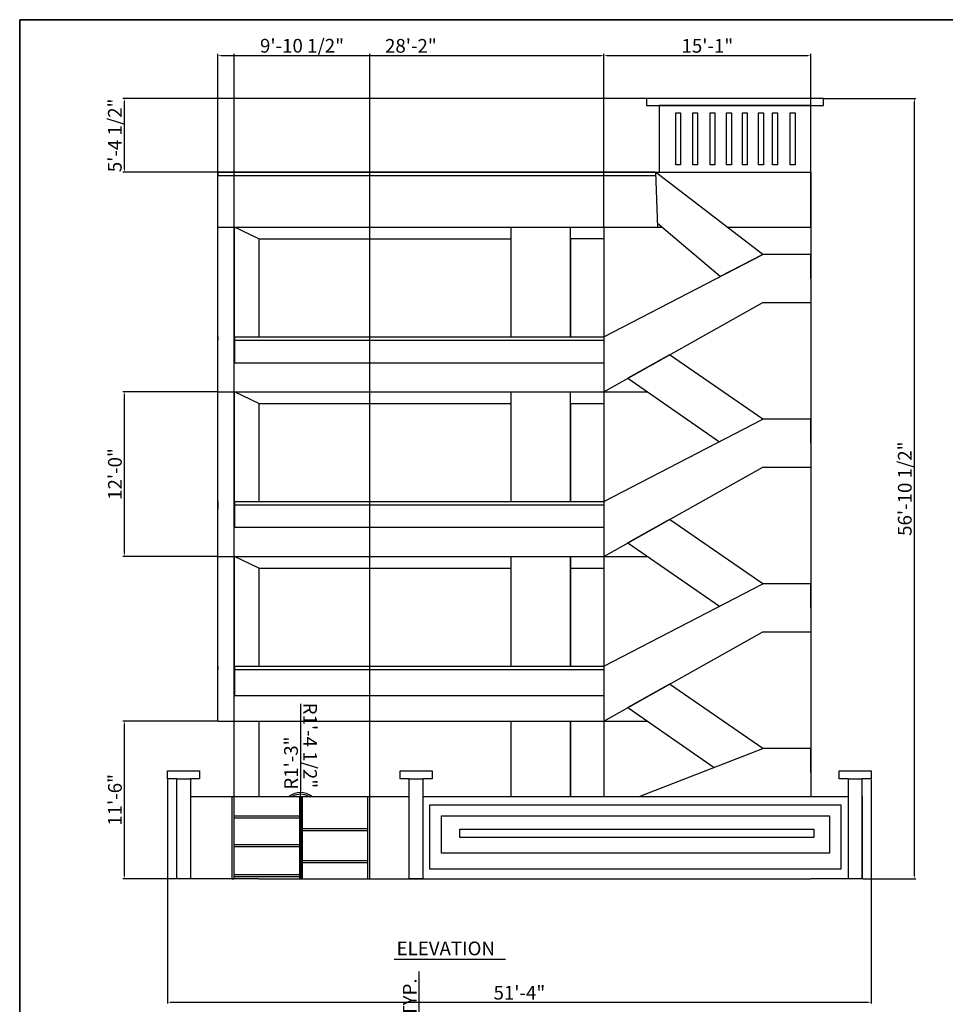
# Model space of a CAD drawing. Units: inches. Extents: x 1266 to 2869, y -408 to 3241.
# Tile 10 of 11: x 1266 to 2076, y 2380 to 3241. Entities that reach past the tile are written whole.
import ezdxf

# ---------------------------------------------------------------- set-up
doc = ezdxf.new("R2010")
doc.units = ezdxf.units.IN
for name, color, linetype, lineweight in [('A-ANNO-DIMS', 2, 'Continuous', 18), ('A-ANNO-TITL', 7, 'Continuous', 25), ('A-ANNO-TTLB', 7, 'Continuous', 35), ('A-ELEV', 7, 'Continuous', 25), ('A-ELEV-GATE', 7, 'Continuous', 25)]:
    doc.layers.add(name, color=color, linetype=linetype, lineweight=lineweight)
doc.styles.get("Standard").update_dxf_attribs({"font": 'arial.ttf'})
doc.dimstyles.new('ISO-25', dxfattribs={"dimtxt": 12, "dimasz": 2.5, "dimexe": 1.25, "dimexo": 0.625, "dimtad": 1, "dimdec": 0, "dimlunit": 3, "dimtxsty": 'Standard', "dimcen": 2.5, "dimadec": 0, "dimazin": 0, "dimtfac": 1, "dimtdec": 0, "dimtmove": 0, "dimatfit": 3, "dimfxl": 1, "dimarcsym": 0})

# ---------------------------------------------------------------- blocks, each defined once
blk = doc.blocks.new('*D53')
at = {"layer": 'A-ANNO-DIMS', "color": 0, "lineweight": -2, "transparency": 16777216}
for p, q in [((1616.02, 2184.29), (1616.02, 2408.76)), ((1611.05, 2184.29), (1617.27, 2184.29)), ((1616.02, 2149.49), (1616.02, 2181.79)), ((1611.05, 2146.99), (1617.27, 2146.99))]:
    blk.add_line(p, q, dxfattribs=at)
at = {"layer": 'A-ANNO-DIMS', "color": 0, "transparency": 16777216}
for points in [[(1615.6, 2181.79), (1616.43, 2181.79), (1616.02, 2184.29)], [(1615.6, 2149.49), (1616.43, 2149.49), (1616.02, 2146.99)]]:
    blk.add_solid(points, dxfattribs=at)
at = {"layer": 'Defpoints', "color": 0, "transparency": 16777216}
for p in [(1610.42, 2184.29), (1616.02, 2184.29), (1610.42, 2146.99)]:
    blk.add_point(p, dxfattribs=at)
at = {"layer": 'A-ANNO-DIMS', "color": 0, "transparency": 16777216, "insert": (1609.18, 2297.78), "char_height": 12, "attachment_point": 5, "rotation": 90}
blk.add_mtext('BEDROOM DR 3\'-1 1/2" TYP.', dxfattribs=at)
blk = doc.blocks.new('*D88')
at = {"layer": 'A-ANNO-DIMS', "color": 0, "lineweight": -2, "transparency": 16777216}
for p, q in [((1395.69, 2576.89), (1395.69, 2380.74)), ((2011.5, 2576.89), (2011.5, 2380.74)), ((1398.19, 2381.99), (2009, 2381.99))]:
    blk.add_line(p, q, dxfattribs=at)
at = {"layer": 'A-ANNO-DIMS', "color": 0, "transparency": 16777216}
for points in [[(1398.19, 2382.41), (1398.19, 2381.57), (1395.69, 2381.99)], [(2009, 2382.41), (2009, 2381.57), (2011.5, 2381.99)]]:
    blk.add_solid(points, dxfattribs=at)
at = {"layer": 'Defpoints', "color": 0, "transparency": 16777216}
for p in [(1395.69, 2577.52), (2011.5, 2577.52), (2011.5, 2381.99)]:
    blk.add_point(p, dxfattribs=at)
at = {"layer": 'A-ANNO-DIMS', "color": 0, "transparency": 16777216, "insert": (1703.6, 2388.74), "char_height": 12, "attachment_point": 5}
blk.add_mtext('51\'-4"', dxfattribs=at)
blk = doc.blocks.new('*D89')
at = {"layer": 'A-ANNO-DIMS', "color": 0, "lineweight": -2, "transparency": 16777216}
for p, q in [((1970.49, 3172.35), (2050.55, 3172.35)), ((2049.3, 2492.46), (2049.3, 3169.85)), ((2004.13, 2489.96), (2050.55, 2489.96))]:
    blk.add_line(p, q, dxfattribs=at)
at = {"layer": 'A-ANNO-DIMS', "color": 0, "transparency": 16777216}
for points in [[(2048.89, 3169.85), (2049.72, 3169.85), (2049.3, 3172.35)], [(2048.89, 2492.46), (2049.72, 2492.46), (2049.3, 2489.96)]]:
    blk.add_solid(points, dxfattribs=at)
at = {"layer": 'Defpoints', "color": 0, "transparency": 16777216}
for p in [(1969.86, 3172.35), (2049.3, 3172.35), (2003.5, 2489.96)]:
    blk.add_point(p, dxfattribs=at)
at = {"layer": 'A-ANNO-DIMS', "color": 0, "transparency": 16777216, "insert": (2042.47, 2831.15), "char_height": 12, "attachment_point": 5, "rotation": 90}
blk.add_mtext('56\'-10 1/2"', dxfattribs=at)
blk = doc.blocks.new('*D90')
at = {"layer": 'A-ANNO-DIMS', "color": 0, "lineweight": -2, "transparency": 16777216}
for p, q in [((1439.69, 3108.58), (1439.69, 3211.4)), ((1442.19, 3210.15), (1775.05, 3210.15)), ((1777.55, 3060.58), (1777.55, 3211.4))]:
    blk.add_line(p, q, dxfattribs=at)
at = {"layer": 'A-ANNO-DIMS', "color": 0, "transparency": 16777216}
for points in [[(1442.19, 3210.57), (1442.19, 3209.73), (1439.69, 3210.15)], [(1775.05, 3210.57), (1775.05, 3209.73), (1777.55, 3210.15)]]:
    blk.add_solid(points, dxfattribs=at)
at = {"layer": 'Defpoints', "color": 0, "transparency": 16777216}
for p in [(1777.55, 3210.15), (1439.69, 3107.96), (1777.55, 3059.96)]:
    blk.add_point(p, dxfattribs=at)
at = {"layer": 'A-ANNO-DIMS', "color": 0, "transparency": 16777216, "insert": (1608.62, 3216.9), "char_height": 12, "attachment_point": 5}
blk.add_mtext('28\'-2"', dxfattribs=at)
blk = doc.blocks.new('*D91')
at = {"layer": 'A-ANNO-DIMS', "color": 0, "lineweight": -2, "transparency": 16777216}
for p, q in [((1777.55, 3060.58), (1777.55, 3211.4)), ((1780.05, 3210.15), (1956.19, 3210.15)), ((1958.69, 3060.58), (1958.69, 3211.4))]:
    blk.add_line(p, q, dxfattribs=at)
at = {"layer": 'A-ANNO-DIMS', "color": 0, "transparency": 16777216}
for points in [[(1780.05, 3210.57), (1780.05, 3209.73), (1777.55, 3210.15)], [(1956.19, 3210.57), (1956.19, 3209.73), (1958.69, 3210.15)]]:
    blk.add_solid(points, dxfattribs=at)
at = {"layer": 'Defpoints', "color": 0, "transparency": 16777216}
for p in [(1958.69, 3210.15), (1777.55, 3059.96), (1958.69, 3059.96)]:
    blk.add_point(p, dxfattribs=at)
at = {"layer": 'A-ANNO-DIMS', "color": 0, "transparency": 16777216, "insert": (1868.12, 3216.9), "char_height": 12, "attachment_point": 5}
blk.add_mtext('15\'-1"', dxfattribs=at)
blk = doc.blocks.new('*D92')
at = {"layer": 'A-ANNO-DIMS', "color": 0, "lineweight": -2, "transparency": 16777216}
for p, q in [((1439.07, 2915.96), (1356.64, 2915.96)), ((1357.89, 2774.46), (1357.89, 2913.46)), ((1439.07, 2771.96), (1356.64, 2771.96))]:
    blk.add_line(p, q, dxfattribs=at)
at = {"layer": 'A-ANNO-DIMS', "color": 0, "transparency": 16777216}
for points in [[(1357.48, 2913.46), (1358.31, 2913.46), (1357.89, 2915.96)], [(1357.48, 2774.46), (1358.31, 2774.46), (1357.89, 2771.96)]]:
    blk.add_solid(points, dxfattribs=at)
at = {"layer": 'Defpoints', "color": 0, "transparency": 16777216}
for p in [(1357.89, 2915.96), (1439.69, 2915.96), (1439.69, 2771.96)]:
    blk.add_point(p, dxfattribs=at)
at = {"layer": 'A-ANNO-DIMS', "color": 0, "transparency": 16777216, "insert": (1351.14, 2843.96), "char_height": 12, "attachment_point": 5, "rotation": 90}
blk.add_mtext('12\'-0"', dxfattribs=at)
blk = doc.blocks.new('*D93')
at = {"layer": 'A-ANNO-DIMS', "color": 0, "lineweight": -2, "transparency": 16777216}
for p, q in [((1969.24, 3172.35), (1356.64, 3172.35)), ((1357.89, 3110.46), (1357.89, 3169.85)), ((1822.02, 3107.96), (1356.64, 3107.96))]:
    blk.add_line(p, q, dxfattribs=at)
at = {"layer": 'A-ANNO-DIMS', "color": 0, "transparency": 16777216}
for points in [[(1357.48, 3169.85), (1358.31, 3169.85), (1357.89, 3172.35)], [(1357.48, 3110.46), (1358.31, 3110.46), (1357.89, 3107.96)]]:
    blk.add_solid(points, dxfattribs=at)
at = {"layer": 'Defpoints', "color": 0, "transparency": 16777216}
for p in [(1357.89, 3172.35), (1969.86, 3172.35), (1822.65, 3107.96)]:
    blk.add_point(p, dxfattribs=at)
at = {"layer": 'A-ANNO-DIMS', "color": 0, "transparency": 16777216, "insert": (1351.06, 3140.15), "char_height": 12, "attachment_point": 5, "rotation": 90}
blk.add_mtext('5\'-4 1/2"', dxfattribs=at)
blk = doc.blocks.new('*D94')
at = {"layer": 'A-ANNO-DIMS', "color": 0, "lineweight": -2, "transparency": 16777216}
for p, q in [((1439.07, 2627.96), (1356.64, 2627.96)), ((1357.89, 2492.46), (1357.89, 2625.46)), ((1403.07, 2489.96), (1356.64, 2489.96))]:
    blk.add_line(p, q, dxfattribs=at)
at = {"layer": 'A-ANNO-DIMS', "color": 0, "transparency": 16777216}
for points in [[(1357.48, 2625.46), (1358.31, 2625.46), (1357.89, 2627.96)], [(1357.48, 2492.46), (1358.31, 2492.46), (1357.89, 2489.96)]]:
    blk.add_solid(points, dxfattribs=at)
at = {"layer": 'Defpoints', "color": 0, "transparency": 16777216}
for p in [(1357.89, 2627.96), (1439.69, 2627.96), (1403.69, 2489.96)]:
    blk.add_point(p, dxfattribs=at)
at = {"layer": 'A-ANNO-DIMS', "color": 0, "transparency": 16777216, "insert": (1351.14, 2558.96), "char_height": 12, "attachment_point": 5, "rotation": 90}
blk.add_mtext('11\'-6"', dxfattribs=at)
blk = doc.blocks.new('*D95')
at = {"layer": 'A-ANNO-DIMS', "color": 0, "lineweight": -2, "transparency": 16777216}
for p, q in [((1454.05, 2562.58), (1454.05, 3211.4)), ((1456.55, 3210.15), (1570.14, 3210.15)), ((1572.64, 2562.58), (1572.64, 3211.4))]:
    blk.add_line(p, q, dxfattribs=at)
at = {"layer": 'A-ANNO-DIMS', "color": 0, "transparency": 16777216}
for points in [[(1456.55, 3210.57), (1456.55, 3209.73), (1454.05, 3210.15)], [(1570.14, 3210.57), (1570.14, 3209.73), (1572.64, 3210.15)]]:
    blk.add_solid(points, dxfattribs=at)
at = {"layer": 'Defpoints', "color": 0, "transparency": 16777216}
for p in [(1572.64, 3210.15), (1454.05, 2561.96), (1572.64, 2561.96)]:
    blk.add_point(p, dxfattribs=at)
at = {"layer": 'A-ANNO-DIMS', "color": 0, "transparency": 16777216, "insert": (1513.34, 3216.98), "char_height": 12, "attachment_point": 5}
blk.add_mtext('9\'-10 1/2"', dxfattribs=at)
blk = doc.blocks.new('*D102')
at = {"layer": 'A-ANNO-DIMS', "color": 0, "lineweight": -2, "transparency": 16777216}
for p, q in [((1512.02, 2642.88), (1512.02, 2567.79)), ((1512.02, 2548.71), (1512.02, 2565.29))]:
    blk.add_line(p, q, dxfattribs=at)
at = {"layer": 'A-ANNO-DIMS', "color": 0, "transparency": 16777216}
blk.add_solid([(1512.44, 2567.79), (1511.61, 2567.79), (1512.02, 2565.29)], dxfattribs=at)
at = {"layer": 'Defpoints', "color": 0, "transparency": 16777216}
for p in [(1512.02, 2565.29), (1512.02, 2548.71)]:
    blk.add_point(p, dxfattribs=at)
at = {"layer": 'A-ANNO-DIMS', "color": 0, "transparency": 16777216, "insert": (1518.85, 2606.59), "char_height": 12, "attachment_point": 5, "rotation": 270.00131}
blk.add_mtext('R1\'-4 1/2"', dxfattribs=at)
blk = doc.blocks.new('*D103')
at = {"layer": 'A-ANNO-DIMS', "color": 0, "lineweight": -2, "transparency": 16777216}
for p, q in [((1512.08, 2613.48), (1512.08, 2566.34)), ((1512.08, 2548.82), (1512.08, 2563.84))]:
    blk.add_line(p, q, dxfattribs=at)
at = {"layer": 'A-ANNO-DIMS', "color": 0, "transparency": 16777216}
blk.add_solid([(1511.66, 2566.34), (1512.49, 2566.34), (1512.08, 2563.84)], dxfattribs=at)
at = {"layer": 'Defpoints', "color": 0, "transparency": 16777216}
for p in [(1512.08, 2563.84), (1512.08, 2548.82)]:
    blk.add_point(p, dxfattribs=at)
at = {"layer": 'A-ANNO-DIMS', "color": 0, "transparency": 16777216, "insert": (1505.32, 2591.16), "char_height": 12, "attachment_point": 5, "rotation": 89.99844}
blk.add_mtext('R1\'-3"', dxfattribs=at)

msp = doc.modelspace()

# ---------------------------------------------------------------- linework, layer by layer
at = {"layer": 'A-ANNO-TITL'}
msp.add_line((1594.11, 2419.79), (1691.47, 2419.79), dxfattribs=at)
at = {"layer": 'A-ANNO-TTLB'}
msp.add_lwpolyline([(1266.23, 3241.34), (2868.62, 3241.34), (2868.62, 986.84), (1266.23, 986.84)], close=True, dxfattribs=at)
at = {"layer": 'A-ELEV'}
for p, q in [((1969.86, 3172.35), (1814.99, 3172.35)), ((1814.99, 3172.35), (1814.99, 3166.35)), ((1969.86, 3170.35), (1969.86, 3172.35)), ((1969.86, 3168.35), (1969.86, 3170.35)), ((1814.99, 3166.35), (1829.61, 3166.35)), ((1958.69, 3166.35), (1825.8, 3166.35)), ((1825.8, 3166.35), (1825.8, 3107.96)), ((1829.61, 3166.35), (1958.69, 3166.35)), ((1958.69, 3107.96), (1958.69, 3166.35)), ((1958.69, 3166.35), (1969.86, 3166.35)), ((1969.86, 3166.35), (1969.86, 3168.35)), ((1439.69, 3107.96), (1822.65, 3107.96)), ((1439.69, 2627.96), (1439.69, 3107.96)), ((1439.69, 3107.96), (1439.69, 3104.96)), ((1439.69, 3104.96), (1822.76, 3104.98)), ((1916.69, 3035.96), (1822.65, 3107.96)), ((1822.65, 3107.96), (1958.69, 3107.96)), ((1822.65, 3107.96), (1824.53, 3059.96)), ((1958.69, 3107.96), (1958.69, 2921.96)), ((1439.69, 3059.96), (1828.01, 3059.96)), ((1475.69, 3049.53), (1454.14, 3059.96)), ((1454.14, 2963.96), (1454.14, 3059.96)), ((1696.19, 3059.96), (1696.19, 2963.96)), ((1748.19, 2963.96), (1748.19, 3059.96)), ((1777.55, 3059.96), (1777.55, 2561.96)), ((1879.39, 3016.66), (1824.41, 3062.99)), ((1885.34, 3059.96), (1958.69, 3059.96)), ((1475.69, 3049.53), (1696.19, 3049.53)), ((1475.69, 3049.53), (1475.69, 2963.96)), ((1696.19, 3049.53), (1696.19, 2963.96)), ((1748.19, 3049.53), (1748.19, 2963.96)), ((1777.55, 3049.53), (1748.19, 3049.53)), ((1777.55, 2963.96), (1916.69, 3035.96)), ((1916.69, 3035.96), (1879.39, 3016.66)), ((1958.69, 3035.96), (1916.69, 3035.96)), ((1958.69, 3035.96), (1916.69, 3035.96)), ((1958.69, 3032.96), (1958.69, 3035.96)), ((1958.69, 3014.96), (1958.69, 3032.96)), ((1777.55, 2915.96), (1916.69, 2993.96)), ((1916.69, 2993.96), (1958.69, 2993.96)), ((1916.69, 2993.96), (1958.69, 2993.96)), ((1439.69, 2963.96), (1439.69, 2960.96)), ((1454.14, 2963.96), (1777.55, 2963.96)), ((1454.14, 2963.96), (1454.14, 2941.23)), ((1958.69, 2963.96), (1958.69, 2777.96)), ((1454.14, 2960.96), (1777.55, 2960.96)), ((1835.11, 2948.22), (1798.47, 2927.68)), ((1916.69, 2891.96), (1835.11, 2948.22)), ((1454.14, 2941.23), (1777.55, 2941.23)), ((1798.47, 2927.68), (1878.65, 2872.27)), ((1439.69, 2915.96), (1777.55, 2915.96)), ((1475.69, 2905.53), (1454.14, 2915.96)), ((1454.14, 2819.96), (1454.14, 2915.96)), ((1696.19, 2915.96), (1696.19, 2819.96)), ((1748.19, 2819.96), (1748.19, 2915.96)), ((1777.55, 2915.96), (1815.44, 2915.95)), ((1475.69, 2905.53), (1475.69, 2819.96)), ((1475.69, 2905.53), (1696.19, 2905.53)), ((1696.19, 2905.53), (1696.19, 2819.96)), ((1748.19, 2905.53), (1748.19, 2819.96)), ((1748.19, 2905.53), (1777.55, 2905.53)), ((1777.55, 2819.96), (1916.69, 2891.96)), ((1958.69, 2891.96), (1916.69, 2891.96)), ((1958.69, 2891.96), (1916.69, 2891.96)), ((1958.69, 2891.96), (1916.69, 2891.96)), ((1958.69, 2888.96), (1958.69, 2891.96)), ((1958.69, 2870.96), (1958.69, 2888.96)), ((1777.55, 2771.96), (1916.69, 2849.96)), ((1916.69, 2849.96), (1958.69, 2849.96)), ((1916.69, 2849.96), (1958.69, 2849.96)), ((1916.69, 2849.96), (1958.69, 2849.96)), ((1439.69, 2819.96), (1439.69, 2815.37)), ((1439.69, 2819.96), (1439.69, 2816.96)), ((1454.14, 2819.96), (1777.55, 2819.96)), ((1454.14, 2819.96), (1454.14, 2797.47)), ((1454.14, 2816.96), (1777.55, 2816.96)), ((1958.69, 2819.96), (1958.69, 2633.96)), ((1439.69, 2815.37), (1439.69, 2813.37)), ((1835.11, 2804.22), (1798.47, 2783.68)), ((1916.69, 2747.96), (1835.11, 2804.22)), ((1454.14, 2797.47), (1777.55, 2797.47)), ((1798.47, 2783.68), (1878.65, 2728.27)), ((1439.69, 2771.96), (1777.55, 2771.96)), ((1454.14, 2675.96), (1454.14, 2771.96)), ((1475.69, 2761.53), (1454.14, 2771.96)), ((1696.19, 2771.96), (1696.19, 2675.96)), ((1696.19, 2771.96), (1696.19, 2675.96)), ((1748.19, 2771.96), (1748.19, 2675.96)), ((1748.19, 2675.96), (1748.19, 2771.96)), ((1777.55, 2771.96), (1815.44, 2771.95)), ((1475.69, 2761.53), (1696.19, 2761.53)), ((1475.69, 2761.53), (1475.69, 2675.96)), ((1748.19, 2761.53), (1777.55, 2761.53)), ((1777.55, 2675.96), (1916.69, 2747.96)), ((1958.69, 2747.96), (1916.69, 2747.96)), ((1958.69, 2747.96), (1916.69, 2747.96)), ((1958.69, 2744.96), (1958.69, 2747.96)), ((1958.69, 2726.96), (1958.69, 2744.96)), ((1777.55, 2627.96), (1916.69, 2705.96)), ((1916.69, 2705.96), (1958.69, 2705.96)), ((1916.69, 2705.96), (1958.69, 2705.96)), ((1439.69, 2675.96), (1439.69, 2672.96)), ((1454.14, 2675.96), (1777.55, 2675.96)), ((1454.14, 2675.96), (1454.14, 2650.2)), ((1454.14, 2672.96), (1777.55, 2672.96)), ((1958.69, 2675.96), (1958.69, 2561.96)), ((1835.11, 2660.22), (1798.47, 2639.68)), ((1916.69, 2603.96), (1835.11, 2660.22)), ((1454.14, 2650.2), (1777.55, 2650.2)), ((1798.47, 2639.68), (1874.09, 2587.42)), ((1439.69, 2627.96), (1777.55, 2627.96)), ((1475.69, 2627.96), (1475.69, 2561.96)), ((1696.19, 2627.96), (1696.19, 2561.96)), ((1696.19, 2627.96), (1696.19, 2561.96)), ((1748.19, 2627.96), (1748.19, 2561.96)), ((1748.19, 2561.96), (1748.19, 2627.96)), ((1777.55, 2627.96), (1815.44, 2627.95)), ((1808.47, 2561.96), (1916.69, 2603.96)), ((1958.69, 2603.96), (1916.69, 2603.96)), ((1958.69, 2600.96), (1958.69, 2603.96)), ((1958.69, 2582.96), (1958.69, 2600.96)), ((1916.69, 2561.96), (1958.69, 2561.96)), ((1475.69, 2489.96), (1958.69, 2489.96))]:
    msp.add_line(p, q, dxfattribs=at)
for points in [[(1840.48, 3159.91), (1844.66, 3159.91), (1844.66, 3114.4), (1840.48, 3114.4)], [(1840.48, 3159.91), (1844.66, 3159.91), (1844.66, 3114.4), (1840.48, 3114.4)], [(1855.28, 3159.91), (1859.46, 3159.91), (1859.46, 3114.4), (1855.28, 3114.4)], [(1870.54, 3159.91), (1874.72, 3159.91), (1874.72, 3114.4), (1870.54, 3114.4)], [(1885, 3159.91), (1889.18, 3159.91), (1889.18, 3114.4), (1885, 3114.4)], [(1898.9, 3159.91), (1903.08, 3159.91), (1903.08, 3114.4), (1898.9, 3114.4)], [(1913.02, 3159.91), (1917.2, 3159.91), (1917.2, 3114.4), (1913.02, 3114.4)], [(1925.22, 3159.91), (1929.4, 3159.91), (1929.4, 3114.4), (1925.22, 3114.4)], [(1940.7, 3159.91), (1944.88, 3159.91), (1944.88, 3114.4), (1940.7, 3114.4)]]:
    msp.add_lwpolyline(points, close=True, dxfattribs=at)
at = {"layer": 'A-ELEV-GATE'}
for p, q in [((1395.69, 2578.52), (1395.69, 2584.52)), ((1395.69, 2584.52), (1403.69, 2584.52)), ((1403.69, 2584.52), (1415.69, 2584.52)), ((1415.69, 2584.52), (1423.69, 2584.52)), ((1423.69, 2584.52), (1423.69, 2578.52)), ((1599.15, 2577.52), (1599.15, 2584.52)), ((1599.15, 2584.52), (1607.15, 2584.52)), ((1607.15, 2584.52), (1619.15, 2584.52)), ((1619.15, 2584.52), (1627.15, 2584.52)), ((1627.15, 2584.52), (1627.15, 2577.52)), ((1983.5, 2577.52), (1983.5, 2584.52)), ((1983.5, 2584.52), (1991.5, 2584.52)), ((1991.5, 2584.52), (2003.5, 2584.52)), ((2003.5, 2584.52), (2011.5, 2584.52)), ((2011.5, 2584.52), (2011.5, 2577.52)), ((1395.69, 2577.52), (1395.69, 2578.52)), ((1403.69, 2577.52), (1395.69, 2577.52)), ((1403.69, 2561.96), (1403.69, 2577.52)), ((1403.69, 2577.52), (1415.69, 2577.52)), ((1415.69, 2577.52), (1415.69, 2489.96)), ((1423.69, 2577.52), (1415.69, 2577.52)), ((1423.69, 2578.52), (1423.69, 2577.52)), ((1607.15, 2577.52), (1599.15, 2577.52)), ((1607.15, 2561.96), (1607.15, 2577.52)), ((1607.15, 2577.52), (1619.15, 2577.52)), ((1619.15, 2577.52), (1619.15, 2489.96)), ((1627.15, 2577.52), (1619.15, 2577.52)), ((1991.5, 2577.52), (1983.5, 2577.52)), ((1991.5, 2577.52), (1991.5, 2489.96)), ((1991.5, 2577.52), (2003.5, 2577.52)), ((2003.5, 2489.96), (2003.5, 2577.52)), ((2003.5, 2577.52), (2003.5, 2577.52)), ((2011.5, 2577.52), (2003.5, 2577.52)), ((1403.69, 2549.96), (1403.69, 2561.96)), ((1415.69, 2561.96), (1607.15, 2561.96)), ((1452.05, 2561.96), (1452.05, 2489.96)), ((1454.05, 2489.96), (1454.05, 2561.96)), ((1454.05, 2561.96), (1570.64, 2561.96)), ((1511.34, 2489.96), (1511.34, 2561.96)), ((1511.34, 2561.96), (1511.34, 2561.96)), ((1511.34, 2561.96), (1512.34, 2561.96)), ((1512.34, 2561.96), (1512.34, 2489.96)), ((1512.34, 2561.96), (1513.34, 2561.96)), ((1513.34, 2561.96), (1513.34, 2489.96)), ((1570.64, 2561.96), (1570.64, 2489.96)), ((1572.64, 2489.96), (1572.64, 2561.96)), ((1572.64, 2561.96), (1572.64, 2561.96)), ((1607.15, 2549.96), (1607.15, 2561.96)), ((1619.15, 2561.96), (1991.5, 2561.96)), ((2003.5, 2561.96), (2003.5, 2489.96)), ((1403.69, 2489.96), (1403.69, 2549.96)), ((1607.15, 2489.96), (1607.15, 2549.96)), ((1454.05, 2545.05), (1511.34, 2545.05)), ((1511.34, 2543.05), (1454.05, 2543.05)), ((1511.34, 2545.05), (1511.34, 2543.05)), ((1513.34, 2533.93), (1570.64, 2533.93)), ((1570.64, 2531.93), (1513.34, 2531.93)), ((1454.05, 2520), (1511.34, 2520)), ((1511.34, 2518), (1454.05, 2518)), ((1513.34, 2505.81), (1570.64, 2505.81)), ((1570.64, 2503.81), (1513.34, 2503.81)), ((1415.69, 2489.96), (1403.69, 2489.96)), ((1475.69, 2489.96), (1415.69, 2489.96)), ((1452.05, 2489.96), (1454.05, 2489.96)), ((1454.05, 2493.7), (1511.34, 2493.7)), ((1511.34, 2491.7), (1454.05, 2491.7)), ((1512.34, 2489.96), (1511.34, 2489.96)), ((1570.64, 2489.96), (1572.64, 2489.96)), ((1619.15, 2489.96), (1607.15, 2489.96)), ((2003.5, 2489.96), (1958.69, 2489.96))]:
    msp.add_line(p, q, dxfattribs=at)
for points in [[(1625.27, 2554.62), (1985.01, 2554.62), (1985.01, 2498.34), (1625.27, 2498.34)], [(1635.45, 2544.91), (1975.14, 2544.91), (1975.14, 2512.37), (1635.45, 2512.37)], [(1651.49, 2533.34), (1961.41, 2533.34), (1961.41, 2525.94), (1651.49, 2525.94)]]:
    msp.add_lwpolyline(points, close=True, dxfattribs=at)
for centre, radius, start, end in [((1512.02, 2548.71), 16.58, 53.04014, 126.95986), ((1512.08, 2548.82), 15.02, 60.9942, 119.0058)]:
    msp.add_arc(centre, radius, start, end, dxfattribs=at)

# ---------------------------------------------------------------- texts
at = {"layer": 'A-ANNO-TITL', "insert": (1596.12, 2435.03), "char_height": 12, "attachment_point": 1}
msp.add_mtext_dynamic_manual_height_columns('ELEVATION', width=415.5917, gutter_width=12.5, heights=[0], dxfattribs=at)

# ---------------------------------------------------------------- dimensions: what is measured, and where the dimension line sits
at = {"layer": 'A-ANNO-DIMS'}
for base, p1, p2, picture, middle in [((1572.64, 3210.15), (1454.05, 2561.96), (1572.64, 2561.96), '*D95', (1513.34, 3216.98)), ((1777.55, 3210.15), (1439.69, 3107.96), (1777.55, 3059.96), '*D90', (1608.62, 3216.9)), ((1958.69, 3210.15), (1777.55, 3059.96), (1958.69, 3059.96), '*D91', (1868.12, 3216.9)), ((2011.5, 2381.99), (1395.69, 2577.52), (2011.5, 2577.52), '*D88', (1703.6, 2388.74))]:
    dim = msp.add_linear_dim(base=base, p1=p1, p2=p2, dimstyle='ISO-25', override={"dimdec": 1, "dimlfac": 1, "dimrnd": 0, "dimzin": 1, "dimdsep": 46, "dimlunit": 4, "dimfrac": 2}, dxfattribs=at)
    dim.commit()
    dim.dimension.update_dxf_attribs({"geometry": picture, "text_midpoint": middle})
for base, p1, p2, picture, middle in [((1357.89, 3172.35), (1822.65, 3107.96), (1969.86, 3172.35), '*D93', (1351.06, 3140.15)), ((2049.3, 3172.35), (2003.5, 2489.96), (1969.86, 3172.35), '*D89', (2042.47, 2831.15)), ((1357.89, 2915.96), (1439.69, 2771.96), (1439.69, 2915.96), '*D92', (1351.14, 2843.96)), ((1357.89, 2627.96), (1403.69, 2489.96), (1439.69, 2627.96), '*D94', (1351.14, 2558.96))]:
    dim = msp.add_linear_dim(base=base, p1=p1, p2=p2, angle=90, dimstyle='ISO-25', override={"dimdec": 1, "dimlfac": 1, "dimrnd": 0, "dimzin": 1, "dimdsep": 46, "dimlunit": 4, "dimfrac": 2}, dxfattribs=at)
    dim.commit()
    dim.dimension.update_dxf_attribs({"geometry": picture, "text_midpoint": middle})
for center, mpoint, picture, middle in [((1512.02, 2548.71), (1512.02, 2565.29), '*D102', (1518.85, 2606.59)), ((1512.08, 2548.82), (1512.08, 2563.84), '*D103', (1505.32, 2591.16))]:
    dim = msp.add_radius_dim(center=center, mpoint=mpoint, dimstyle='ISO-25', override={"dimdec": 1, "dimlfac": 1, "dimrnd": 0, "dimzin": 1, "dimdsep": 46, "dimlunit": 4, "dimfrac": 2}, dxfattribs=at)
    dim.commit()
    dim.dimension.update_dxf_attribs({"geometry": picture, "text_midpoint": middle})
dim = msp.add_linear_dim(base=(1616.02, 2184.29), p1=(1610.42, 2146.99), p2=(1610.42, 2184.29), angle=90, text='BEDROOM DR <> TYP.', dimstyle='ISO-25', override={"dimdec": 1, "dimlfac": 1, "dimrnd": 0, "dimzin": 1, "dimdsep": 46, "dimlunit": 4, "dimfrac": 2}, dxfattribs=at)
dim.commit()
dim.dimension.update_dxf_attribs({"geometry": '*D53', "text_midpoint": (1609.18, 2297.78)})

doc.saveas('drawing.dxf')
